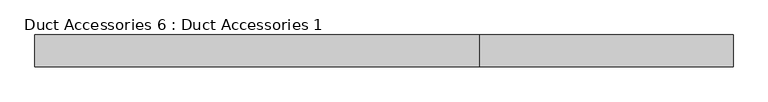
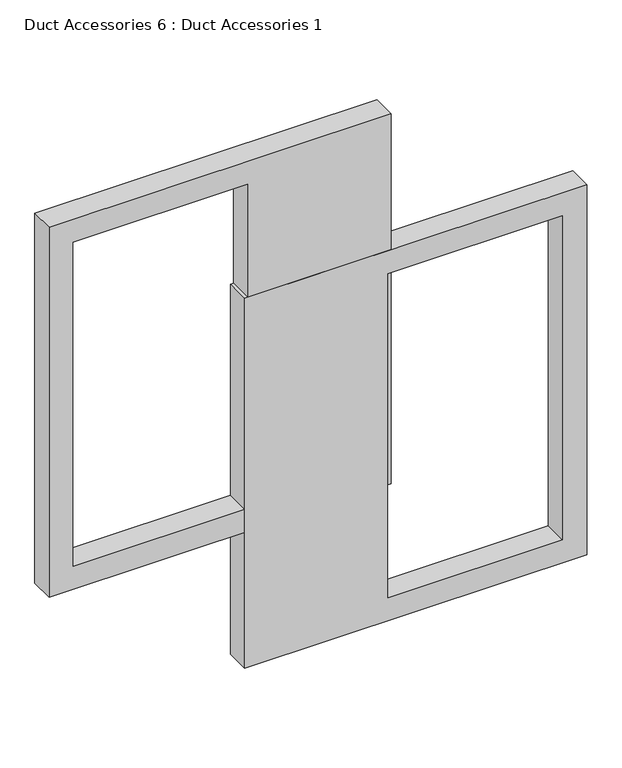
"""IFC4 building model written with IfcOpenShell, lengths in millimetres: damper geometry, Duct Accessories 6 : Duct Accessories 1."""

from ifc_helpers import new_model, si_unit, frame, origin, place, context, project, spatial, polyline, outline, extrude, source, transform, mapped, element, save


def duct_accessories_6_duct_accessories_1_9dfa8ad6(model_context):
    return source(origin(), model_context, "Body", "SweptSolid", [
        extrude(outline(polyline([(22830.3403114, -12928.36893), (21611.1403114, -12928.36893), (21611.1403114, -11861.56893), (22830.3403114, -11861.56893), (22830.3403114, -12928.36893)]), holes=[polyline([(22754.1403114, -12480.9324751), (22754.1403114, -11937.76893), (21687.3403114, -11937.76893), (21687.3403114, -12480.9324751), (22754.1403114, -12480.9324751)])]), frame((0.0, -447.4934478, 0.0), z_axis=(0.0, 1.0, 0.0), x_axis=(0.0, 0.0, 1.0)), (0.0, 0.0, 1.0), 76.2),
        extrude(outline(polyline([(23277.7767663, -12471.5606701), (23277.7767663, -13538.3606701), (22058.5767663, -13538.3606701), (22058.5767663, -12471.5606701), (23277.7767663, -12471.5606701)]), holes=[polyline([(23201.5767663, -12918.997125), (22134.7767663, -12918.997125), (22134.7767663, -13462.1606701), (23201.5767663, -13462.1606701), (23201.5767663, -12918.997125)])]), frame((0.0, -447.4934478, 0.0), z_axis=(0.0, 1.0, 0.0), x_axis=(0.0, 0.0, 1.0)), (0.0, 0.0, 1.0), 76.2),
    ])


if __name__ == "__main__":
    model = new_model("IFC4")
    model_context = context("Model", 3, world=origin())
    ifc_project = project(units=[si_unit("LENGTHUNIT", "METRE", prefix="MILLI")], contexts=[model_context])
    site = spatial("IfcSite", under=ifc_project)
    building = spatial("IfcBuilding", under=site)
    placement = place(None, origin())
    duct_accessories_6_duct_accessories_1_shape = duct_accessories_6_duct_accessories_1_9dfa8ad6(model_context)
    element("IfcDamper", 1, ObjectType="Duct Accessories 6 : Duct Accessories 1", at=placement, inside=building, context=model_context, shape_type="MappedRepresentation", body=[
        mapped(duct_accessories_6_duct_accessories_1_shape, transform((0.0, 0.0, 0.0), x_axis=(1.0, 0.0, 0.0), y_axis=(0.0, 1.0, 0.0), z_axis=(0.0, 0.0, 1.0))),
    ])
    save(model, "model.ifc")

# Revit data of these elements
# Element 1 (IfcDamper, "Duct Accessories 6 : Duct Accessories 1")
#   Materials on its faces: "border"
# Materials
#   "border": class "Generic", colour RGB 144 144 144, transparency 0, Cost = 0
